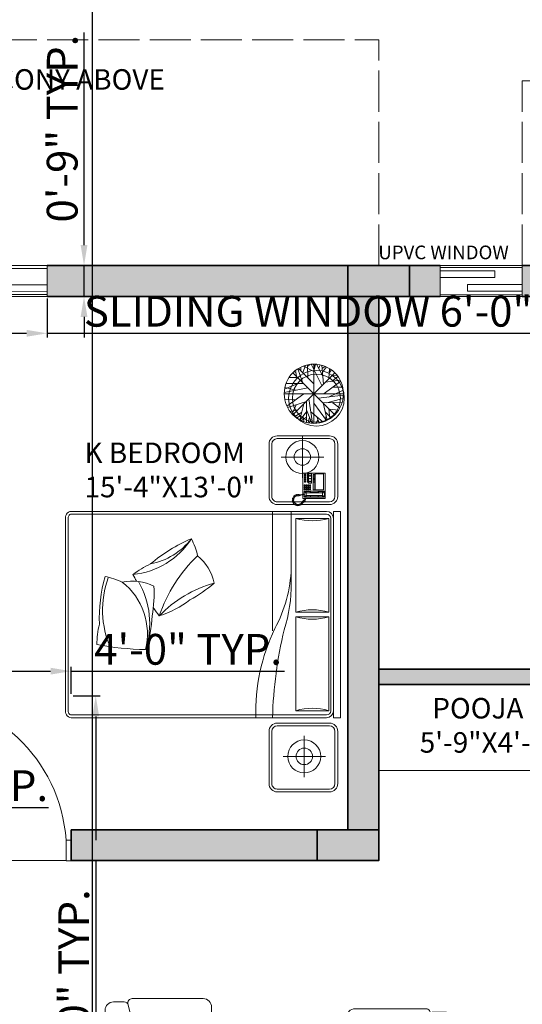
# Model space of a CAD drawing. Units: millimetres. Extents: x 595116 to 630915, y 909473 to 920225.
# Tile 123 of 134: x 629490 to 629637, y 919742 to 920030. Entities that reach past the tile are written whole.
import ezdxf

# ---------------------------------------------------------------- set-up
doc = ezdxf.new("R2010")
doc.units = ezdxf.units.MM
doc.linetypes.add('ACAD_ISO02W100', pattern=[15, 12, -3])
for name, color, linetype, lineweight in [('A-AREA-IDEN', 7, 'Continuous', 20), ('A-FLOR-OVHD', 253, 'ACAD_ISO02W100', 13), ('A-FURN', 32, 'Continuous', 18), ('A-WALL', 1, 'Continuous', 35), ('A-WALL-PATT', 8, 'Continuous', 13), ('Column', 6, 'Continuous', 35), ('Dimension', 3, 'Continuous', 18), ('Doors', 31, 'Continuous', 20), ('L-PLNT', 85, 'Continuous', 13), ('Text', 7, 'Continuous', 18), ('Windows', 33, 'Continuous', 18)]:
    doc.layers.add(name, color=color, linetype=linetype, lineweight=lineweight)
doc.styles.get("Standard").update_dxf_attribs({"font": 'arial.ttf'})
doc.dimstyles.new('ISO-25', dxfattribs={"dimtxt": 9, "dimasz": 6, "dimexe": 1.25, "dimexo": 0.625, "dimtad": 1, "dimlunit": 4, "dimtxsty": 'Standard', "dimcen": 2.5, "dimadec": 0, "dimazin": 0, "dimtfac": 1, "dimtmove": 0, "dimatfit": 3, "dimfxl": 1, "dimarcsym": 0})

# ---------------------------------------------------------------- blocks, each defined once
blk = doc.blocks.new('KWD')
for points in [[(629753.63, 919957.93), (629752.54, 919957.93), (629752.54, 919953.43), (629753.63, 919953.43)], [(629787.45, 919957.93), (629787.45, 919953.43), (629788.54, 919953.43), (629788.54, 919957.93)]]:
    blk.add_lwpolyline(points, close=True)
blk.add_lwpolyline([(629753.63, 919921.79), (629753.63, 919955.68), (629754.13, 919955.68), (629754.13, 919921.8)])
blk.add_arc((629753.64, 919955.68), 33.88, 269.99, 356.196)
blk = doc.blocks.new('A$C356F0359')
for p, q in [((0.4398, 1.9801), (0.0598, 1.9801)), ((0.4398, 1.9601), (0.0598, 1.9601)), ((0.5489, 2), (2.0492, 2)), ((0.5489, 1.9489), (0.5489, 2)), ((2.0492, 1.9489), (0.5489, 1.9489)), ((2.0492, 1.9489), (2.0492, 2)), ((2.5283, 1.9801), (2.1483, 1.9801)), ((2.5283, 1.9601), (2.1483, 1.9601)), ((-0.0002, 1.9201), (-0.0002, 1.5401)), ((0.0198, 1.9201), (0.0198, 1.5401)), ((0.1539, 1.5681), (0.1539, 1.8777)), ((0.2725, 1.8879), (0.2702, 1.8856)), ((0.2702, 1.8856), (0.2702, 1.7279)), ((0.2725, 1.8879), (0.4531, 1.8879)), ((0.3913, 1.8753), (0.277, 1.8753)), ((0.277, 1.8753), (0.277, 1.8147)), ((0.3913, 1.8147), (0.3913, 1.8753)), ((0.4016, 1.8787), (0.4062, 1.8845)), ((0.4016, 1.7404), (0.4016, 1.8787)), ((0.4062, 1.881), (0.405, 1.8765)), ((0.405, 1.8765), (0.4153, 1.8662)), ((0.405, 1.8765), (0.405, 1.8456)), ((0.4062, 1.8845), (0.4405, 1.8845)), ((0.4108, 1.8833), (0.4062, 1.881)), ((0.4108, 1.8833), (0.4382, 1.8833)), ((0.4165, 1.8685), (0.4108, 1.8833)), ((0.4153, 1.8662), (0.4165, 1.8685)), ((0.4153, 1.8147), (0.4153, 1.8662)), ((0.4325, 1.8685), (0.4165, 1.8685)), ((0.4325, 1.8685), (0.4382, 1.8833)), ((0.4336, 1.8662), (0.4325, 1.8685)), ((0.4439, 1.8765), (0.4336, 1.8662)), ((0.4336, 1.8147), (0.4336, 1.8662)), ((0.4382, 1.8833), (0.4428, 1.881)), ((0.4405, 1.8845), (0.4462, 1.8787)), ((0.4428, 1.881), (0.4439, 1.8765)), ((0.4439, 1.8765), (0.4439, 1.8456)), ((0.4462, 1.8787), (0.4462, 1.7416)), ((0.4531, 1.8879), (0.4553, 1.8856)), ((0.4553, 1.8856), (0.4553, 1.7279)), ((0.4798, 1.5401), (0.4798, 1.9201)), ((0.4998, 1.5401), (0.4998, 1.9201)), ((0.5489, 1.8977), (0.5489, 0.0512)), ((0.5689, 1.8977), (0.5689, 0.0512)), ((1.998, 1.9289), (0.6001, 1.9289)), ((2.0292, 0.0512), (2.0292, 1.8977)), ((2.0492, 0.0512), (2.0492, 1.8977)), ((2.0883, 1.9201), (2.0883, 1.5401)), ((2.1083, 1.9201), (2.1083, 1.5401)), ((2.3306, 1.5822), (2.3306, 1.8917)), ((2.5683, 1.5401), (2.5683, 1.9201)), ((2.5883, 1.5401), (2.5883, 1.9201)), ((0.277, 1.8147), (0.3913, 1.8147)), ((0.3913, 1.8125), (0.2816, 1.8125)), ((0.2816, 1.8125), (0.2816, 1.801)), ((0.2816, 1.801), (0.3913, 1.801)), ((0.2907, 1.8125), (0.2907, 1.801)), ((0.2999, 1.8125), (0.2999, 1.801)), ((0.309, 1.8125), (0.309, 1.801)), ((0.3182, 1.8125), (0.3182, 1.801)), ((0.3273, 1.8125), (0.3273, 1.801)), ((0.3365, 1.8125), (0.3365, 1.801)), ((0.3913, 1.801), (0.3913, 1.8125)), ((0.405, 1.8456), (0.4073, 1.8399)), ((0.4073, 1.8399), (0.4108, 1.8342)), ((0.4108, 1.8342), (0.4119, 1.8262)), ((0.4108, 1.785), (0.4119, 1.793)), ((0.4119, 1.8262), (0.4119, 1.8147)), ((0.4119, 1.793), (0.4119, 1.8147)), ((0.4153, 1.8147), (0.4153, 1.753)), ((0.4336, 1.8147), (0.4336, 1.753)), ((0.4382, 1.8342), (0.4371, 1.8262)), ((0.4371, 1.8262), (0.4371, 1.8147)), ((0.4371, 1.793), (0.4371, 1.8147)), ((0.4382, 1.785), (0.4371, 1.793)), ((0.4416, 1.8399), (0.4382, 1.8342)), ((0.4439, 1.8456), (0.4416, 1.8399)), ((0.3052, 1.7226), (0.0051, 1.7226)), ((0.2702, 1.7279), (0.2725, 1.7256)), ((0.4244, 1.7256), (0.2725, 1.7256)), ((0.277, 1.7885), (0.277, 1.7679)), ((0.3445, 1.7885), (0.277, 1.7885)), ((0.277, 1.7679), (0.3445, 1.7679)), ((0.2782, 1.7622), (0.2782, 1.7576)), ((0.2896, 1.7622), (0.2782, 1.7622)), ((0.2782, 1.7576), (0.2896, 1.7576)), ((0.2782, 1.745), (0.2896, 1.745)), ((0.2782, 1.7382), (0.2782, 1.745)), ((0.2896, 1.7382), (0.2782, 1.7382)), ((0.2885, 1.7862), (0.2885, 1.7827)), ((0.2919, 1.7862), (0.2885, 1.7862)), ((0.2885, 1.7827), (0.2919, 1.7827)), ((0.2919, 1.7736), (0.2885, 1.7736)), ((0.2885, 1.7736), (0.2885, 1.7702)), ((0.2885, 1.7702), (0.2919, 1.7702)), ((0.2896, 1.7576), (0.2896, 1.7622)), ((0.2896, 1.745), (0.2896, 1.7382)), ((0.2919, 1.7827), (0.2919, 1.7862)), ((0.2919, 1.7702), (0.2919, 1.7736)), ((0.2942, 1.7622), (0.2942, 1.7576)), ((0.3056, 1.7622), (0.2942, 1.7622)), ((0.2942, 1.7576), (0.3056, 1.7576)), ((0.2942, 1.745), (0.3056, 1.745)), ((0.2942, 1.7382), (0.2942, 1.745)), ((0.3056, 1.7382), (0.2942, 1.7382)), ((0.3056, 1.7576), (0.3056, 1.7622)), ((0.3056, 1.745), (0.3056, 1.7382)), ((0.3125, 1.7862), (0.309, 1.7862)), ((0.309, 1.7862), (0.309, 1.7827)), ((0.309, 1.7827), (0.3125, 1.7827)), ((0.3125, 1.7736), (0.309, 1.7736)), ((0.309, 1.7736), (0.309, 1.7702)), ((0.309, 1.7702), (0.3125, 1.7702)), ((0.3102, 1.7622), (0.3102, 1.7576)), ((0.3216, 1.7622), (0.3102, 1.7622)), ((0.3102, 1.7576), (0.3216, 1.7576)), ((0.3102, 1.745), (0.3216, 1.745)), ((0.3102, 1.7382), (0.3102, 1.745)), ((0.3216, 1.7382), (0.3102, 1.7382)), ((0.3125, 1.7827), (0.3125, 1.7862)), ((0.3125, 1.7702), (0.3125, 1.7736)), ((0.3216, 1.7576), (0.3216, 1.7622)), ((0.3216, 1.745), (0.3216, 1.7382)), ((0.3376, 1.7622), (0.3262, 1.7622)), ((0.3262, 1.7622), (0.3262, 1.7576)), ((0.3262, 1.7576), (0.3376, 1.7576)), ((0.3262, 1.7382), (0.3262, 1.745)), ((0.3262, 1.745), (0.3376, 1.745)), ((0.3376, 1.7382), (0.3262, 1.7382)), ((0.333, 1.7862), (0.3296, 1.7862)), ((0.3296, 1.7862), (0.3296, 1.7827)), ((0.3296, 1.7827), (0.333, 1.7827)), ((0.333, 1.7736), (0.3296, 1.7736)), ((0.3296, 1.7736), (0.3296, 1.7702)), ((0.3296, 1.7702), (0.333, 1.7702)), ((0.333, 1.7827), (0.333, 1.7862)), ((0.333, 1.7702), (0.333, 1.7736)), ((0.3376, 1.7576), (0.3376, 1.7622)), ((0.3376, 1.745), (0.3376, 1.7382)), ((0.3445, 1.7679), (0.3445, 1.7885)), ((0.3548, 1.7759), (0.3548, 1.7827)), ((0.3548, 1.7827), (0.3639, 1.7827)), ((0.3639, 1.7759), (0.3548, 1.7759)), ((0.3548, 1.7633), (0.3548, 1.7702)), ((0.3548, 1.7702), (0.3639, 1.7702)), ((0.3639, 1.7633), (0.3548, 1.7633)), ((0.3548, 1.7564), (0.3639, 1.7564)), ((0.3548, 1.7496), (0.3548, 1.7564)), ((0.3639, 1.7496), (0.3548, 1.7496)), ((0.3548, 1.737), (0.3548, 1.7439)), ((0.3548, 1.7439), (0.3639, 1.7439)), ((0.3639, 1.737), (0.3548, 1.737)), ((0.3639, 1.7827), (0.3639, 1.7759)), ((0.3639, 1.7702), (0.3639, 1.7633)), ((0.3639, 1.7564), (0.3639, 1.7496)), ((0.3639, 1.7439), (0.3639, 1.737)), ((0.3685, 1.7827), (0.3776, 1.7827)), ((0.3685, 1.7759), (0.3685, 1.7827)), ((0.3776, 1.7759), (0.3685, 1.7759)), ((0.3685, 1.7633), (0.3685, 1.7702)), ((0.3685, 1.7702), (0.3776, 1.7702)), ((0.3776, 1.7633), (0.3685, 1.7633)), ((0.3685, 1.7564), (0.3776, 1.7564)), ((0.3685, 1.7496), (0.3685, 1.7564)), ((0.3776, 1.7496), (0.3685, 1.7496)), ((0.3685, 1.737), (0.3685, 1.7439)), ((0.3685, 1.7439), (0.3776, 1.7439)), ((0.3776, 1.737), (0.3685, 1.737)), ((0.3776, 1.7827), (0.3776, 1.7759)), ((0.3776, 1.7702), (0.3776, 1.7633)), ((0.3776, 1.7564), (0.3776, 1.7496)), ((0.3776, 1.7439), (0.3776, 1.737)), ((0.3822, 1.7759), (0.3822, 1.7827)), ((0.3822, 1.7827), (0.3913, 1.7827)), ((0.3913, 1.7759), (0.3822, 1.7759)), ((0.3822, 1.7633), (0.3822, 1.7702)), ((0.3822, 1.7702), (0.3913, 1.7702)), ((0.3913, 1.7633), (0.3822, 1.7633)), ((0.3822, 1.7576), (0.3913, 1.7576)), ((0.3822, 1.7507), (0.3822, 1.7576)), ((0.3913, 1.7507), (0.3822, 1.7507)), ((0.3822, 1.7439), (0.3913, 1.7439)), ((0.3822, 1.737), (0.3822, 1.7439)), ((0.3913, 1.737), (0.3822, 1.737)), ((0.3913, 1.7827), (0.3913, 1.7759)), ((0.3913, 1.7702), (0.3913, 1.7633)), ((0.3913, 1.7576), (0.3913, 1.7507)), ((0.3913, 1.7439), (0.3913, 1.737)), ((0.4073, 1.7347), (0.4016, 1.7404)), ((0.405, 1.7736), (0.4073, 1.7793)), ((0.405, 1.7427), (0.405, 1.7736)), ((0.405, 1.7427), (0.4153, 1.753)), ((0.4062, 1.7382), (0.405, 1.7427)), ((0.4108, 1.7359), (0.4062, 1.7382)), ((0.4073, 1.7793), (0.4108, 1.785)), ((0.4234, 1.7347), (0.4073, 1.7347)), ((0.4165, 1.7507), (0.4108, 1.7359)), ((0.4108, 1.7359), (0.4234, 1.7359)), ((0.4153, 1.753), (0.4165, 1.7507)), ((0.4325, 1.7507), (0.4165, 1.7507)), ((0.4233, 1.7393), (0.4235, 1.7294)), ((0.4268, 1.7393), (0.4233, 1.7393)), ((0.4235, 1.7294), (0.4263, 1.7179)), ((0.4274, 1.7301), (0.4268, 1.7393)), ((0.427, 1.7359), (0.4382, 1.7359)), ((0.4405, 1.7347), (0.4271, 1.7347)), ((0.429, 1.7227), (0.4274, 1.7301)), ((0.4531, 1.7256), (0.4284, 1.7256)), ((0.4318, 1.7119), (0.429, 1.7227)), ((0.4336, 1.753), (0.4325, 1.7507)), ((0.4325, 1.7507), (0.4382, 1.7359)), ((0.4439, 1.7427), (0.4336, 1.753)), ((0.4416, 1.7793), (0.4382, 1.785)), ((0.4382, 1.7359), (0.4428, 1.7382)), ((0.4462, 1.7416), (0.4405, 1.7347)), ((0.4439, 1.7736), (0.4416, 1.7793)), ((0.4428, 1.7382), (0.4439, 1.7427)), ((0.4439, 1.7427), (0.4439, 1.7736)), ((0.4553, 1.7279), (0.4531, 1.7256)), ((0.4622, 1.7459), (0.4553, 1.7484)), ((0.4553, 1.7439), (0.4604, 1.7425)), ((0.4604, 1.7425), (0.465, 1.7388)), ((0.4654, 1.7427), (0.4622, 1.7459)), ((0.465, 1.7388), (0.4662, 1.7372)), ((0.4678, 1.7405), (0.4654, 1.7427)), ((0.4662, 1.7372), (0.4686, 1.7374)), ((0.4686, 1.7374), (0.4662, 1.735)), ((0.4662, 1.735), (0.4755, 1.7268)), ((0.4721, 1.7421), (0.4678, 1.7405)), ((0.4741, 1.7401), (0.4721, 1.7421)), ((0.4725, 1.7366), (0.4741, 1.7401)), ((0.4753, 1.7388), (0.4725, 1.7366)), ((0.4783, 1.7356), (0.4753, 1.7388)), ((0.4755, 1.7268), (0.4906, 1.7139)), ((0.4759, 1.729), (0.4783, 1.7356)), ((0.4821, 1.7322), (0.4759, 1.729)), ((0.4874, 1.7272), (0.4821, 1.7322)), ((0.4862, 1.7199), (0.4874, 1.7272)), ((0.4914, 1.7231), (0.4862, 1.7199)), ((0.4958, 1.7185), (0.4914, 1.7231)), ((0.494, 1.7135), (0.4958, 1.7185)), ((2.4819, 1.7366), (2.1818, 1.7366)), ((0.4263, 1.7179), (0.429, 1.707)), ((0.427, 1.697), (0.4265, 1.6915)), ((0.4265, 1.6915), (0.4332, 1.6903)), ((0.4332, 1.6903), (0.4267, 1.6864)), ((0.4267, 1.6864), (0.4272, 1.6801)), ((0.4295, 1.6996), (0.427, 1.697)), ((0.4272, 1.6801), (0.4346, 1.6794)), ((0.4346, 1.6794), (0.4281, 1.6744)), ((0.4281, 1.6744), (0.4311, 1.669)), ((0.429, 1.707), (0.4288, 1.701)), ((0.4288, 1.701), (0.4295, 1.6996)), ((0.4311, 1.669), (0.4381, 1.6704)), ((0.4325, 1.7063), (0.4318, 1.7119)), ((0.4323, 1.7003), (0.4325, 1.7063)), ((0.4364, 1.6973), (0.4323, 1.7003)), ((0.4381, 1.6704), (0.4348, 1.6639)), ((0.4348, 1.6639), (0.4383, 1.6598)), ((0.4355, 1.6919), (0.4364, 1.6973)), ((0.4367, 1.6774), (0.4355, 1.6919)), ((0.4455, 1.6663), (0.4367, 1.6774)), ((0.4383, 1.6598), (0.4436, 1.6637)), ((0.4436, 1.6637), (0.4427, 1.6575)), ((0.4427, 1.6575), (0.4471, 1.6547)), ((0.4577, 1.6598), (0.4455, 1.6663)), ((0.4471, 1.6547), (0.4526, 1.6593)), ((0.4526, 1.6593), (0.4519, 1.6517)), ((0.4519, 1.6517), (0.4568, 1.6503)), ((0.4568, 1.6503), (0.4598, 1.6565)), ((0.4716, 1.6586), (0.4577, 1.6598)), ((0.4598, 1.6565), (0.4626, 1.6503)), ((0.4626, 1.6503), (0.4665, 1.6498)), ((0.4665, 1.6498), (0.4681, 1.6565)), ((0.4681, 1.6565), (0.4707, 1.6491)), ((0.4707, 1.6491), (0.4751, 1.6503)), ((0.485, 1.6644), (0.4716, 1.6586)), ((0.4751, 1.6503), (0.4753, 1.6565)), ((0.4753, 1.6565), (0.4806, 1.6519)), ((0.4806, 1.6519), (0.4843, 1.6538)), ((0.4843, 1.6538), (0.4836, 1.6607)), ((0.4836, 1.6607), (0.4885, 1.6547)), ((0.4952, 1.6744), (0.485, 1.6644)), ((0.4885, 1.6547), (0.4922, 1.6579)), ((0.4922, 1.6579), (0.4894, 1.6642)), ((0.4894, 1.6642), (0.4959, 1.6614)), ((0.4908, 1.7135), (0.4984, 1.6917)), ((0.501, 1.7142), (0.494, 1.7135)), ((0.4984, 1.6917), (0.4952, 1.6744)), ((0.4957, 1.6704), (0.5024, 1.6683)), ((0.4989, 1.6642), (0.4957, 1.6704)), ((0.4959, 1.6614), (0.4989, 1.6642)), ((0.4964, 1.7047), (0.5031, 1.7072)), ((0.5038, 1.7049), (0.4964, 1.7047)), ((0.5042, 1.673), (0.4987, 1.6792)), ((0.4987, 1.6792), (0.5058, 1.679)), ((0.5005, 1.695), (0.5054, 1.6996)), ((0.5068, 1.695), (0.5005, 1.695)), ((0.5008, 1.6871), (0.5079, 1.6892)), ((0.5068, 1.6836), (0.5008, 1.6871)), ((0.5031, 1.7072), (0.501, 1.7142)), ((0.5024, 1.6683), (0.5042, 1.673)), ((0.5054, 1.6996), (0.5038, 1.7049)), ((0.5058, 1.679), (0.5068, 1.6836)), ((0.5079, 1.6892), (0.5068, 1.695)), ((0.0598, 1.5001), (0.4398, 1.5001)), ((0.0598, 1.4801), (0.4398, 1.4801)), ((2.1483, 1.5001), (2.5283, 1.5001)), ((2.1483, 1.4801), (2.5283, 1.4801)), ((0.6001, 0.02), (1.998, 0.02)), ((0.6001, 0), (1.998, 0))]:
    blk.add_line(p, q)
at = {"linetype": 'ByBlock'}
for p, q in [((0.6001, 1.9147), (1.282, 1.9147)), ((0.6001, 1.6759), (0.6001, 1.9147)), ((1.282, 1.9147), (1.282, 1.6759)), ((1.3161, 1.9147), (1.998, 1.9147)), ((1.3161, 1.6759), (1.3161, 1.9147)), ((1.998, 1.9147), (1.998, 1.6759)), ((1.282, 1.6759), (0.6001, 1.6759)), ((1.998, 1.6759), (1.3161, 1.6759)), ((1.0687, 1.6418), (0.5489, 1.6418)), ((1.4185, 1.5053), (0.5489, 1.5053))]:
    blk.add_line(p, q, dxfattribs=at)
for centre in [(0.1539, 1.7226), (2.3306, 1.7366)]:
    blk.add_circle(centre, 0.12, dxfattribs=at)
for centre in [(2.3306, 1.7366), (0.1539, 1.7226)]:
    blk.add_circle(centre, 0.06)
for centre, radius, start, end in [((0.0598, 1.9201), 0.06, 90, 180), ((0.0598, 1.9201), 0.04, 90, 180), ((0.4398, 1.9201), 0.06, 0, 90), ((0.4398, 1.9201), 0.04, 0, 90), ((0.6001, 1.8977), 0.0512, 90, 180), ((1.998, 1.8977), 0.0512, 0, 90), ((2.1483, 1.9201), 0.06, 90, 180), ((2.1483, 1.9201), 0.04, 90, 180), ((2.5283, 1.9201), 0.06, 0, 90), ((2.5283, 1.9201), 0.04, 0, 90), ((0.6001, 1.8977), 0.0312, 90, 180), ((1.998, 1.8977), 0.0312, 0, 90), ((0.0598, 1.5401), 0.06, 180, 270), ((0.0598, 1.5401), 0.04, 180, 270), ((0.4398, 1.5401), 0.04, 270, 0), ((0.4398, 1.5401), 0.06, 270, 0), ((2.1483, 1.5401), 0.06, 180, 270), ((2.1483, 1.5401), 0.04, 180, 270), ((2.5283, 1.5401), 0.06, 270, 0), ((2.5283, 1.5401), 0.04, 270, 0), ((1.1471, 0.7332), 0.3575, 102.47819, 140.46254), ((1.9086, 1.3124), 0.8697, 195.33601, 226.41927), ((0.3249, 0.4335), 0.9879, 28.49711, 41.05657), ((0.9965, 0.4273), 0.548, 103.20343, 117.03623), ((1.6529, 1.7059), 1.0798, 223.63057, 251.4288), ((0.4451, 0.4375), 0.5655, 5.33912, 57.68949), ((0.4517, 0.5274), 0.4879, 10.69865, 52.68638), ((1.8195, 1.3719), 1.1652, 203.06416, 220.32086), ((0.5617, 0.4344), 0.7874, 18.35266, 36.68512), ((1.1372, -0.3434), 0.9879, 80.06073, 92.62018), ((-0.021, 2.4319), 2.1977, 305.29657, 307.24182), ((1.5949, 0.9312), 0.734, 205.25901, 216.93514), ((1.4135, 0.487), 0.3575, 154.0418, 192.02615), ((1.3641, 0.0041), 0.6085, 71.81005, 120.13512), ((1.44, 0.1186), 0.4774, 76.18494, 142.00166), ((1.2836, -0.1573), 0.7874, 69.91627, 88.24873), ((-0.6432, 0.628), 2.1977, 349.48843, 358.80544), ((-0.021, 2.4319), 2.1977, 297.92482, 299.3793), ((1.5595, 0.1789), 0.548, 154.76704, 168.59984), ((1.3312, 1.4107), 1.1652, 254.62778, 271.88448), ((1.2647, 0.9578), 0.6885, 250.29361, 293.6414), ((1.5368, 0.9609), 0.734, 256.82263, 268.49876), ((0.5943, 0.0454), 0.0458, 172.75992, 277.24008), ((0.5943, 0.0454), 0.0258, 172.75992, 277.24008), ((2.0038, 0.0454), 0.0458, 262.75992, 7.24008), ((2.0038, 0.0454), 0.0258, 262.75992, 7.24008)]:
    blk.add_arc(centre, radius, start, end)
for centre, radius, start, end in [((0.1906, 1.7953), 0.4265, 343.73979, 16.26021), ((1.6914, 1.7953), 0.4265, 163.73979, 196.26021), ((0.9067, 1.7953), 0.4265, 343.73979, 16.26021), ((2.4075, 1.7953), 0.4265, 163.73979, 196.26021), ((0.9303, 0.657), 0.9853, 61.43285, 88.12613), ((1.0826, 0.5712), 1.0706, 72.19663, 90.74184), ((2.1368, 4.5996), 3.0955, 256.42012, 268.37887), ((2.0056, 2.7745), 1.3903, 244.24266, 271.79845)]:
    blk.add_arc(centre, radius, start, end, dxfattribs=at)
blk = doc.blocks.new('SOFA')
for p, q in [((629543.7, 919743.59), (629522.89, 919743.59)), ((629522.89, 919743.59), (629543.7, 919743.59)), ((629520.59, 919742.63), (629517.45, 919742.63)), ((629517.45, 919742.63), (629520.59, 919742.63)), ((629521.79, 919741.7), (629521.7, 919742.06)), ((629521.7, 919742.06), (629523.2, 919736.06)), ((629546.16, 919741.12), (629546.16, 919739.22)), ((629546.16, 919741.12), (629546.16, 919737.29)), ((629588.11, 919740.62), (629608.91, 919740.62)), ((629588.11, 919740.62), (629608.91, 919740.62)), ((629514.98, 919740.17), (629514.98, 919695.65)), ((629514.98, 919695.65), (629514.98, 919740.17)), ((629547.17, 919738.01), (629547.17, 919695.65)), ((629547.17, 919738.01), (629547.17, 919695.65)), ((629585.64, 919738.15), (629585.64, 919734.33)), ((629585.64, 919736.25), (629585.64, 919738.15)), ((629610.11, 919739.09), (629608.61, 919733.09)), ((629610.11, 919739.09), (629610.02, 919738.73)), ((629611.21, 919739.66), (629614.36, 919739.66)), ((629611.21, 919739.66), (629614.36, 919739.66)), ((629523.2, 919736.06), (629523.2, 919695.65)), ((629523.2, 919695.65), (629523.2, 919736.06)), ((629523.2, 919695.65), (629523.2, 919736.06)), ((629544.93, 919736.06), (629523.2, 919736.06)), ((629523.2, 919736.06), (629523.53, 919736.06)), ((629523.2, 919736.06), (629523.53, 919736.06)), ((629523.53, 919736.06), (629523.53, 919695.65)), ((629523.53, 919736.06), (629523.53, 919695.65)), ((629523.53, 919736.06), (629523.53, 919695.65)), ((629584.64, 919735.04), (629584.64, 919712.53)), ((629584.64, 919712.53), (629584.64, 919735.04)), ((629616.82, 919737.2), (629616.82, 919710.3)), ((629616.82, 919737.2), (629616.82, 919710.3)), ((629586.87, 919733.09), (629608.61, 919733.09)), ((629608.28, 919733.09), (629608.61, 919733.09)), ((629608.28, 919714.4), (629608.28, 919733.09)), ((629608.28, 919733.09), (629608.28, 919714.4)), ((629608.61, 919733.09), (629608.61, 919714.4)), ((629608.61, 919733.09), (629608.61, 919714.4)), ((629556.25, 919728.06), (629556.25, 919687.01)), ((629556.25, 919687.01), (629556.25, 919728.06)), ((629576.77, 919728.06), (629556.25, 919728.06)), ((629556.25, 919728.06), (629576.77, 919728.06)), ((629559.82, 919728), (629559.82, 919727.13)), ((629561.06, 919728), (629561.06, 919725.63)), ((629562.29, 919728), (629562.29, 919724.5)), ((629563.52, 919728), (629563.52, 919723.63)), ((629564.75, 919728), (629564.75, 919722.96)), ((629565.98, 919728), (629565.98, 919722.42)), ((629567.19, 919727.97), (629567.19, 919721.68)), ((629568.42, 919727.08), (629568.42, 919720.54)), ((629576.77, 919687.01), (629576.77, 919728.06)), ((629576.77, 919728.06), (629576.77, 919687.01)), ((629569.65, 919725.8), (629569.65, 919718.67)), ((629569.65, 919725.8), (629569.65, 919718.67)), ((629570.88, 919723.75), (629570.88, 919716.49)), ((629570.88, 919716.49), (629570.88, 919723.75)), ((629572.12, 919720.99), (629572.12, 919714.94)), ((629573.35, 919718.86), (629573.35, 919713.74)), ((629547.17, 919715.59), (629514.98, 919715.59)), ((629574.58, 919717.12), (629574.58, 919712.78)), ((629575.81, 919715.64), (629575.81, 919712.02)), ((629586.87, 919714.4), (629608.61, 919714.4)), ((629608.61, 919714.4), (629608.28, 919714.4)), ((629610.09, 919708.48), (629608.61, 919714.4)), ((629557.33, 919712.4), (629557.33, 919707.56)), ((629557.33, 919707.56), (629557.33, 919712.4)), ((629585.64, 919709.42), (629585.64, 919713.17)), ((629558.57, 919711.23), (629558.57, 919706.97)), ((629559.8, 919710.18), (629559.8, 919706.31)), ((629561.03, 919709.25), (629561.03, 919705.57)), ((629585.64, 919709.42), (629585.64, 919711.32)), ((629610.02, 919708.77), (629610.09, 919708.48)), ((629562.26, 919708.41), (629562.26, 919704.73)), ((629563.49, 919707.66), (629563.49, 919703.8)), ((629564.72, 919706.99), (629564.72, 919702.74)), ((629565.96, 919706.31), (629565.96, 919701.75)), ((629588.11, 919706.95), (629608.89, 919706.95)), ((629608.89, 919706.95), (629588.11, 919706.95)), ((629611.21, 919707.83), (629611.48, 919707.83)), ((629611.48, 919707.83), (629611.21, 919707.83)), ((629611.48, 919707.83), (629614.36, 919707.83)), ((629614.36, 919707.83), (629611.48, 919707.83)), ((629567.19, 919705.56), (629567.19, 919701.12)), ((629568.42, 919704.73), (629568.42, 919700.78)), ((629569.65, 919703.81), (629569.65, 919700.45)), ((629570.88, 919702.8), (629570.88, 919699.98)), ((629572.12, 919701.68), (629572.12, 919699.37)), ((629573.35, 919700.43), (629573.35, 919698.59)), ((629574.58, 919699.04), (629574.58, 919697.6)), ((629575.81, 919697.48), (629575.81, 919696.34)), ((629575.81, 919697.48), (629575.81, 919696.34)), ((629547.17, 919695.06), (629514.98, 919695.06)), ((629514.98, 919695.06), (629514.98, 919670.42)), ((629514.98, 919670.42), (629514.98, 919695.06)), ((629514.98, 919695.06), (629515.44, 919695.06)), ((629515.6, 919695.04), (629546.55, 919695.04)), ((629523.2, 919695.06), (629523.2, 919674.53)), ((629523.2, 919674.53), (629523.2, 919695.04)), ((629523.2, 919674.53), (629523.2, 919695.04)), ((629523.2, 919695.04), (629523.53, 919695.04)), ((629523.2, 919695.04), (629523.53, 919695.04)), ((629523.53, 919695.04), (629523.53, 919695.11)), ((629523.53, 919695.04), (629523.53, 919695.11)), ((629523.53, 919695.06), (629523.53, 919674.53)), ((629523.53, 919695.04), (629523.53, 919674.53)), ((629523.53, 919695.04), (629523.53, 919674.53)), ((629524.14, 919695.04), (629523.53, 919695.04)), ((629524.14, 919695.04), (629523.53, 919695.04)), ((629546.71, 919695.06), (629547.17, 919695.06)), ((629547.17, 919695.06), (629547.17, 919672.66)), ((629547.17, 919695.06), (629547.17, 919672.66)), ((629588.11, 919692.76), (629608.89, 919692.76)), ((629608.89, 919692.76), (629588.11, 919692.76)), ((629611.21, 919691.88), (629611.48, 919691.88)), ((629611.48, 919691.88), (629611.21, 919691.88)), ((629611.48, 919691.88), (629614.36, 919691.88)), ((629614.36, 919691.88), (629611.48, 919691.88)), ((629585.64, 919690.3), (629585.64, 919688.39)), ((629585.64, 919690.3), (629585.64, 919686.55)), ((629610.09, 919691.23), (629608.61, 919685.31)), ((629610.02, 919690.95), (629610.09, 919691.23)), ((629616.82, 919662.52), (629616.82, 919689.42)), ((629616.82, 919662.52), (629616.82, 919689.42)), ((629556.25, 919687.01), (629576.77, 919687.01)), ((629576.77, 919687.01), (629556.25, 919687.01)), ((629584.64, 919664.68), (629584.64, 919687.18)), ((629584.64, 919687.18), (629584.64, 919664.68)), ((629586.87, 919685.31), (629608.61, 919685.31)), ((629608.61, 919685.31), (629608.28, 919685.31)), ((629608.28, 919685.31), (629608.28, 919666.62)), ((629608.28, 919666.62), (629608.28, 919685.31)), ((629608.61, 919666.62), (629608.61, 919685.31)), ((629608.61, 919666.62), (629608.61, 919685.31)), ((629521.72, 919668.61), (629523.2, 919674.53)), ((629544.93, 919674.53), (629523.2, 919674.53)), ((629523.53, 919674.53), (629523.2, 919674.53)), ((629523.53, 919674.53), (629523.2, 919674.53)), ((629546.16, 919669.54), (629546.16, 919673.3)), ((629546.16, 919671.45), (629546.16, 919669.54)), ((629521.72, 919668.61), (629521.79, 919668.89)), ((629520.32, 919667.96), (629517.45, 919667.96)), ((629520.32, 919667.96), (629517.45, 919667.96)), ((629520.59, 919667.96), (629520.32, 919667.96)), ((629520.59, 919667.96), (629520.32, 919667.96)), ((629543.7, 919667.08), (629522.91, 919667.08)), ((629543.7, 919667.08), (629522.91, 919667.08)), ((629585.64, 919661.56), (629585.64, 919665.39)), ((629586.87, 919666.62), (629608.61, 919666.62)), ((629608.28, 919666.62), (629608.61, 919666.62)), ((629610.11, 919660.63), (629608.61, 919666.62)), ((629585.64, 919663.47), (629585.64, 919661.56)), ((629610.11, 919660.63), (629610.02, 919660.99)), ((629611.21, 919660.05), (629614.36, 919660.05)), ((629611.21, 919660.05), (629614.36, 919660.05)), ((629588.11, 919659.1), (629608.91, 919659.1)), ((629588.11, 919659.1), (629608.91, 919659.1))]:
    blk.add_line(p, q)
for centre, radius, start, end in [((629522.89, 919742.36), 1.23, 90, 194.0362), ((629522.89, 919742.36), 1.23, 90, 194.0362), ((629543.7, 919741.12), 2.46, 0, 90), ((629543.7, 919741.12), 2.46, 0, 90), ((629517.45, 919740.17), 2.46, 90, 180), ((629517.45, 919740.17), 2.46, 90, 180), ((629520.59, 919741.4), 1.23, 14.0362, 90), ((629520.59, 919741.4), 1.23, 14.0362, 90), ((629588.11, 919738.15), 2.46, 90, 180), ((629588.11, 919738.15), 2.46, 90, 180), ((629608.91, 919739.39), 1.23, 345.9638, 90), ((629608.91, 919739.39), 1.23, 345.9638, 90), ((629545.94, 919738.01), 1.23, 0, 90), ((629545.94, 919738.01), 1.23, 0, 79.4007), ((629611.21, 919738.43), 1.23, 90, 165.9638), ((629611.21, 919738.43), 1.23, 90, 165.9638), ((629614.36, 919737.2), 2.46, 0, 90), ((629614.36, 919737.2), 2.46, 0, 90), ((629544.93, 919737.29), 1.23, 270, 0), ((629585.87, 919735.04), 1.23, 90, 180), ((629585.87, 919735.04), 1.23, 100.5993, 180), ((629586.87, 919734.33), 1.23, 180, 270), ((629570.11, 919734.3), 12.54, 210.2644, 248.0021), ((629562.37, 919720.03), 9.29, 21.2599, 58.8091), ((629562.37, 919720.03), 9.29, 23.6102, 38.4008), ((629594.57, 919732.56), 25.26, 201.2599, 225.1217), ((629562.42, 919715.26), 7.99, 24.8088, 68.0021), ((629582.84, 919724.7), 14.51, 204.5645, 214.4539), ((629582.84, 919724.7), 14.51, 204.8088, 245.1378), ((629586.87, 919713.17), 1.23, 90, 180), ((629577.93, 919732.79), 28.98, 222.2366, 242.5747), ((629577.93, 919732.79), 28.98, 224.7026, 242.5747), ((629585.87, 919712.53), 1.23, 180, 270), ((629585.87, 919712.53), 1.23, 180, 259.4007), ((629588.11, 919709.42), 2.46, 180, 270), ((629588.11, 919709.42), 2.46, 180, 270), ((629611.21, 919709.06), 1.23, 194.0362, 270), ((629611.21, 919709.06), 1.23, 194.0362, 270), ((629614.36, 919710.3), 2.46, 270, 0), ((629614.36, 919710.3), 2.46, 270, 0), ((629546.11, 919682.25), 27.68, 46.9747, 68.4773), ((629546.11, 919682.25), 27.68, 46.9747, 66.0851), ((629549.56, 919678.1), 32.63, 33.5604, 62.5747), ((629549.56, 919678.1), 32.63, 36.4252, 62.5747), ((629608.89, 919708.18), 1.23, 270, 14.0362), ((629608.89, 919708.18), 1.23, 270, 14.0362), ((629569.57, 919707.39), 6.7, 226.9747, 258.3827), ((629569.57, 919707.39), 6.7, 226.9746, 258.3828), ((629565.49, 919687.55), 13.55, 33.8658, 78.3827), ((629565.49, 919687.55), 13.55, 40.4201, 78.3827), ((629515.6, 919695.65), 0.616, 180, 270), ((629515.6, 919695.65), 0.616, 180, 255.079), ((629523.81, 919695.65), 0.616, 180, 270), ((629523.81, 919695.65), 0.616, 180, 242.2854), ((629523.81, 919695.65), 0.616, 180, 242.2854), ((629524.14, 919695.65), 0.616, 180, 270), ((629524.14, 919695.65), 0.616, 180, 270), ((629524.14, 919695.65), 0.616, 180, 270), ((629546.55, 919695.65), 0.616, 270, 0), ((629546.55, 919695.65), 0.616, 284.921, 0), ((629588.11, 919690.3), 2.46, 90, 180), ((629588.11, 919690.3), 2.46, 90, 180), ((629608.89, 919691.53), 1.23, 345.9638, 90), ((629608.89, 919691.53), 1.23, 345.9638, 90), ((629611.21, 919690.65), 1.23, 90, 165.9638), ((629611.21, 919690.65), 1.23, 90, 165.9638), ((629614.36, 919689.42), 2.46, 0, 90), ((629614.36, 919689.42), 2.46, 0, 90), ((629585.87, 919687.18), 1.23, 90, 180), ((629585.87, 919687.18), 1.23, 100.5993, 180), ((629586.87, 919686.55), 1.23, 180, 270), ((629544.93, 919673.3), 1.23, 0, 90), ((629545.94, 919672.66), 1.23, 270, 0), ((629545.94, 919672.66), 1.23, 280.5993, 0), ((629517.45, 919670.42), 2.46, 180, 270), ((629517.45, 919670.42), 2.46, 180, 270), ((629520.59, 919669.19), 1.23, 270, 345.9638), ((629520.59, 919669.19), 1.23, 270, 345.9638), ((629522.91, 919668.31), 1.23, 165.9638, 270), ((629522.91, 919668.31), 1.23, 165.9638, 270), ((629543.7, 919669.54), 2.46, 270, 0), ((629543.7, 919669.54), 2.46, 270, 0), ((629586.87, 919665.39), 1.23, 90, 180), ((629585.87, 919664.68), 1.23, 180, 270), ((629585.87, 919664.68), 1.23, 180, 259.4007), ((629614.36, 919662.52), 2.46, 270, 0), ((629614.36, 919662.52), 2.46, 270, 0), ((629588.11, 919661.56), 2.46, 180, 270), ((629588.11, 919661.56), 2.46, 180, 270), ((629608.91, 919660.33), 1.23, 270, 14.0362), ((629608.91, 919660.33), 1.23, 270, 14.0362), ((629611.21, 919661.28), 1.23, 194.0362, 270), ((629611.21, 919661.28), 1.23, 194.0362, 270)]:
    blk.add_arc(centre, radius, start, end)
at = {"flags": 9}
for tag in ['XSIZE', 'YSIZE']:
    blk.add_attdef(tag, (629556.25, 919728.06), '', height=0.0205, rotation=270, dxfattribs=at)
blk = doc.blocks.new('POTTED-PLANT')
for p, q in [((5.49, 15.52), (6.28, 17.77)), ((5.61, 17.51), (8.67, 15.94)), ((6.86, 17.38), (7.52, 18.03)), ((6.89, 14.08), (6.86, 17.93)), ((7.9, 18.06), (11.06, 11.86)), ((9.02, 17.38), (8.46, 18.1)), ((8.67, 18.11), (8.67, 0.76)), ((8.74, 16.47), (9.2, 18.06)), ((11.32, 14.57), (9.46, 18.06)), ((10.09, 16.89), (10.53, 17.9)), ((11.52, 12.26), (11.04, 17.77)), ((11.14, 16.82), (12.03, 17.41)), ((11.24, 15.75), (12.36, 17.28)), ((14.75, 15.51), (2.6, 3.36)), ((14.75, 3.36), (2.6, 15.51)), ((2.87, 15.88), (3.4, 15.68)), ((3.32, 16.24), (3.58, 14.57)), ((3.96, 16.73), (5.31, 12.84)), ((4.16, 16.82), (8.64, 12.35)), ((4.85, 16.17), (4.88, 17.22)), ((13.25, 16.79), (13.05, 13.86)), ((13.17, 15.58), (13.86, 16.4)), ((13.91, 13.07), (15.74, 14.51)), ((14.04, 14.8), (15.41, 14.87)), ((4.01, 12.42), (0.12, 10.79)), ((0.57, 12.45), (5.66, 12.45)), ((1.47, 14.18), (3.93, 14.18)), ((16.53, 13.1), (11.7, 9.48)), ((12.05, 12.81), (16.38, 13.4)), ((0, 9.44), (17.35, 9.44)), ((0.04, 9.84), (6.94, 11.18)), ((0.19, 11.28), (3.48, 10.53)), ((0.78, 5.86), (5.74, 9.45)), ((10.02, 8.11), (17.3, 9.03)), ((12.92, 8.47), (17.27, 10.46)), ((14.24, 11.38), (17.09, 11.41)), ((0.22, 7.66), (3.4, 7.75)), ((0.98, 5.47), (6.25, 7.04)), ((3.48, 6.19), (2.31, 3.58)), ((5.79, 6.51), (4.54, 1.82)), ((6.53, 7.26), (6.56, 1.1)), ((7.22, 7.98), (8.31, 0.8)), ((8.67, 6.68), (12.41, 1.65)), ((11.37, 6.74), (12.54, 1.72)), ((11.39, 6.74), (16.97, 6.94)), ((12.49, 6.77), (17.19, 8.01)), ((14.19, 6.81), (16.25, 5.24)), ((3.99, 4.75), (1.72, 4.29)), ((5.1, 3.97), (3.07, 2.83)), ((4.88, 3.09), (3.65, 2.4)), ((6.56, 4.2), (4.67, 1.78)), ((6.56, 4.78), (8.11, 0.84)), ((7.78, 4.2), (11.26, 1.2)), ((11.98, 4.16), (13.78, 2.43)), ((12.26, 2.96), (12, 1.49)), ((13.07, 5.08), (13.35, 2.21)), ((13.22, 4.91), (15.85, 4.62)), ((6.56, 2.6), (5.05, 1.59)), ((5.56, 2.86), (5.79, 1.33)), ((7.45, 2.57), (7.01, 0.97)), ((7.75, 1.82), (7.32, 0.93)), ((9.89, 1.75), (9.23, 0.84)), ((9.53, 2.7), (10.2, 0.97))]:
    blk.add_line(p, q)
for centre, radius in [((8.67, 9.44), 8.67), ((9.43, 8.14), 8.14), ((9.43, 8.14), 7.03)]:
    blk.add_circle(centre, radius)
blk = doc.blocks.new('WIN-SLIDING-6FT')
for p, q in [((0, 0), (0, 9)), ((0, 9), (72, 9)), ((72, 0), (72, 9)), ((0.01, 7.5), (42, 7.41)), ((42, 7.41), (42, 5.41)), ((0, 5.5), (42, 5.41)), ((30, 3.44), (72, 3.35)), ((30, 3.44), (30, 1.44)), ((30, 1.44), (71.99, 1.35)), ((0, 0), (72, 0))]:
    blk.add_line(p, q)
blk.add_lwpolyline([(0, 8.12), (72, 8.12), (72, 0.59), (0, 0.59)], close=True)
blk = doc.blocks.new('WIN-SLIDING-2FT')
for p, q in [((0, 9), (0, 0)), ((0, 9), (24, 9)), ((24, 9), (24, 0)), ((0, 7.5), (16, 7.5)), ((16, 7.5), (16, 5.5)), ((0, 5.5), (16, 5.5)), ((8, 3.5), (24, 3.5)), ((8, 3.5), (8, 1.5)), ((8, 1.5), (24, 1.5)), ((0, 0), (24, 0))]:
    blk.add_line(p, q)
blk.add_lwpolyline([(0, 8.46), (24, 8.46), (24, 0.48), (0, 0.48)], close=True)
blk = doc.blocks.new('COLUMN-RECT-18X9')
h = blk.add_hatch(color=256)
h.dxf.hatch_style = 1
h.paths.add_polyline_path([(18, 9), (0, 9), (0, 0), (18, 0)])
blk.add_lwpolyline([(0, 9), (18, 9), (18, 0), (0, 0)], close=True)
blk = doc.blocks.new('*D162')
at = {"layer": 'Defpoints', "color": 0, "transparency": 16777216}
for p in [(629505.04, 919832.11), (629505.04, 919783.93), (629512.27, 919783.93)]:
    blk.add_point(p, dxfattribs=at)
at = {"layer": 'Dimension', "color": 0, "lineweight": -2, "transparency": 16777216}
for p, q in [((629505.67, 919832.11), (629513.52, 919832.11)), ((629512.27, 919826.11), (629512.27, 919789.93)), ((629505.67, 919783.93), (629513.52, 919783.93)), ((629512.27, 919783.93), (629512.27, 919681.05))]:
    blk.add_line(p, q, dxfattribs=at)
at = {"layer": 'Dimension', "color": 0, "transparency": 16777216}
for points in [[(629511.27, 919826.11), (629513.27, 919826.11), (629512.27, 919832.11)], [(629511.27, 919789.93), (629513.27, 919789.93), (629512.27, 919783.93)]]:
    blk.add_solid(points, dxfattribs=at)
at = {"layer": 'Dimension', "color": 0, "transparency": 16777216, "insert": (629506.99, 919729.49), "char_height": 9, "attachment_point": 5, "rotation": 90}
blk.add_mtext('DOOR 4\'-0" TYP.', dxfattribs=at)
blk = doc.blocks.new('*D163')
at = {"layer": 'Defpoints', "color": 0, "transparency": 16777216}
for p in [(629505.04, 919839.34), (629457.04, 919832.11), (629505.04, 919832.11)]:
    blk.add_point(p, dxfattribs=at)
at = {"layer": 'Dimension', "color": 0, "lineweight": -2, "transparency": 16777216}
for p, q in [((629457.04, 919832.74), (629457.04, 919840.59)), ((629463.04, 919839.34), (629499.04, 919839.34)), ((629505.04, 919832.74), (629505.04, 919840.59)), ((629505.04, 919839.34), (629567.51, 919839.34))]:
    blk.add_line(p, q, dxfattribs=at)
at = {"layer": 'Dimension', "color": 0, "transparency": 16777216}
for points in [[(629463.04, 919840.34), (629463.04, 919838.34), (629457.04, 919839.34)], [(629499.04, 919840.34), (629499.04, 919838.34), (629505.04, 919839.34)]]:
    blk.add_solid(points, dxfattribs=at)
at = {"layer": 'Dimension', "color": 0, "transparency": 16777216, "insert": (629539.28, 919844.56), "char_height": 9, "attachment_point": 5}
blk.add_mtext('4\'-0" TYP.', dxfattribs=at)
blk = doc.blocks.new('*D179')
at = {"layer": 'Defpoints', "color": 0, "transparency": 16777216}
for p in [(629417.05, 919802.7), (629437.23, 919802.7), (629437.23, 919799.48)]:
    blk.add_point(p, dxfattribs=at)
at = {"layer": 'Dimension', "color": 0, "lineweight": -2, "transparency": 16777216}
for p, q in [((629417.05, 919802.07), (629417.05, 919798.23)), ((629437.23, 919802.07), (629437.23, 919798.23)), ((629423.05, 919799.48), (629431.23, 919799.48)), ((629437.23, 919799.48), (629498.49, 919799.48))]:
    blk.add_line(p, q, dxfattribs=at)
at = {"layer": 'Dimension', "color": 0, "transparency": 16777216}
for points in [[(629423.05, 919800.48), (629423.05, 919798.48), (629417.05, 919799.48)], [(629431.23, 919800.48), (629431.23, 919798.48), (629437.23, 919799.48)]]:
    blk.add_solid(points, dxfattribs=at)
at = {"layer": 'Dimension', "color": 0, "transparency": 16777216, "insert": (629470.86, 919804.7), "char_height": 9, "attachment_point": 5}
blk.add_mtext('1\'-8" TYP.', dxfattribs=at)
blk = doc.blocks.new('*D192')
at = {"layer": 'Defpoints', "color": 0, "transparency": 16777216}
for p in [(629426.04, 919948.93), (629498.04, 919948.93), (629498.04, 919938.13)]:
    blk.add_point(p, dxfattribs=at)
at = {"layer": 'Dimension', "color": 0, "lineweight": -2, "transparency": 16777216}
for p, q in [((629426.04, 919948.3), (629426.04, 919936.88)), ((629498.04, 919948.3), (629498.04, 919936.88)), ((629432.04, 919938.13), (629492.04, 919938.13)), ((629498.04, 919938.13), (629672.56, 919938.13))]:
    blk.add_line(p, q, dxfattribs=at)
at = {"layer": 'Dimension', "color": 0, "transparency": 16777216}
for points in [[(629432.04, 919939.13), (629432.04, 919937.13), (629426.04, 919938.13)], [(629492.04, 919939.13), (629492.04, 919937.13), (629498.04, 919938.13)]]:
    blk.add_solid(points, dxfattribs=at)
at = {"layer": 'Dimension', "color": 0, "transparency": 16777216, "insert": (629588.3, 919943.41), "char_height": 9, "attachment_point": 5}
blk.add_mtext('SLIDING WINDOW 6\'-0" TYP.', dxfattribs=at)
blk = doc.blocks.new('*D193')
at = {"layer": 'Defpoints', "color": 0, "transparency": 16777216}
for p in [(629498.04, 919957.93), (629508.84, 919957.93), (629498.04, 919948.93)]:
    blk.add_point(p, dxfattribs=at)
at = {"layer": 'Dimension', "color": 0, "lineweight": -2, "transparency": 16777216}
for p, q in [((629508.84, 919963.93), (629508.84, 920026.04)), ((629498.67, 919957.93), (629510.09, 919957.93)), ((629508.84, 919948.93), (629508.84, 919957.93)), ((629498.67, 919948.93), (629510.09, 919948.93)), ((629508.84, 919942.93), (629508.84, 919936.93))]:
    blk.add_line(p, q, dxfattribs=at)
at = {"layer": 'Dimension', "color": 0, "transparency": 16777216}
for points in [[(629507.84, 919963.93), (629509.84, 919963.93), (629508.84, 919957.93)], [(629507.84, 919942.93), (629509.84, 919942.93), (629508.84, 919948.93)]]:
    blk.add_solid(points, dxfattribs=at)
at = {"layer": 'Dimension', "color": 0, "transparency": 16777216, "insert": (629503.62, 919997.98), "char_height": 9, "attachment_point": 5, "rotation": 90}
blk.add_mtext('0\'-9" TYP.', dxfattribs=at)
blk = doc.blocks.new('*D220')
at = {"layer": 'Defpoints', "color": 0, "transparency": 16777216}
for p in [(629824.95, 920160.76), (629511.27, 919302.01), (629824.95, 919302.01)]:
    blk.add_point(p, dxfattribs=at)
at = {"layer": 'Dimension', "color": 0, "lineweight": -2, "transparency": 16777216}
for p, q in [((629511.27, 919302.63), (629511.27, 920162.01)), ((629517.27, 920160.76), (629818.95, 920160.76)), ((629824.95, 919302.63), (629824.95, 920162.01))]:
    blk.add_line(p, q, dxfattribs=at)
at = {"layer": 'Dimension', "color": 0, "transparency": 16777216}
for points in [[(629517.27, 920161.76), (629517.27, 920159.76), (629511.27, 920160.76)], [(629818.95, 920161.76), (629818.95, 920159.76), (629824.95, 920160.76)]]:
    blk.add_solid(points, dxfattribs=at)
at = {"layer": 'Dimension', "color": 0, "transparency": 16777216, "insert": (629668.11, 920166.03), "char_height": 9, "attachment_point": 5}
blk.add_mtext('26\'-1 1/2"', dxfattribs=at)

msp = doc.modelspace()

# ---------------------------------------------------------------- hatches: boundary and pattern name
at = {"layer": 'A-WALL-PATT'}
h = msp.add_hatch(color=256, dxfattribs=at)
h.dxf.hatch_style = 1
h.paths.add_polyline_path([(629586.041, 919957.928), (629498.041, 919957.928), (629498.041, 919948.928), (629586.041, 919948.928)])
h = msp.add_hatch(color=256, dxfattribs=at)
h.dxf.hatch_style = 1
h.paths.add_polyline_path([(629613.041, 919957.928), (629604.041, 919957.928), (629604.041, 919948.928), (629613.041, 919948.928)])
h = msp.add_hatch(color=256, dxfattribs=at)
h.dxf.hatch_style = 1
h.paths.add_polyline_path([(629685.041, 919957.928), (629637.041, 919957.928), (629637.041, 919948.928), (629685.041, 919948.928)])
h = msp.add_hatch(color=256, dxfattribs=at)
h.dxf.hatch_style = 1
h.paths.add_polyline_path([(629595.041, 919948.928), (629586.041, 919948.928), (629586.041, 919792.928), (629595.041, 919792.928)])
h = msp.add_hatch(color=256, dxfattribs=at)
h.dxf.hatch_style = 1
h.paths.add_polyline_path([(629706.041, 919839.928), (629595.041, 919839.928), (629595.041, 919835.428), (629706.041, 919835.428)])
h = msp.add_hatch(color=256, dxfattribs=at)
h.dxf.hatch_style = 1
h.paths.add_polyline_path([(629577.041, 919792.928), (629505.041, 919792.928), (629505.041, 919783.928), (629577.041, 919783.928)])

# ---------------------------------------------------------------- linework, layer by layer
at = {"layer": 'A-FLOR-OVHD'}
for p, q in [((629393.041, 920023.928), (629595.041, 920023.928)), ((629595.041, 919957.928), (629595.041, 920023.928)), ((629637.041, 920011.928), (629833.541, 920011.928)), ((629637.041, 919957.928), (629637.041, 920011.928))]:
    msp.add_line(p, q, dxfattribs=at)
at = {"layer": 'A-FURN'}
msp.add_line((629595.041, 919810.258), (629664.041, 919810.258), dxfattribs=at)
at = {"layer": 'A-WALL'}
for p, q in [((629498.041, 919957.928), (629613.041, 919957.928)), ((629637.041, 919957.928), (629685.041, 919957.928)), ((629498.041, 919948.928), (629586.041, 919948.928)), ((629586.041, 919948.928), (629586.041, 919792.928)), ((629595.041, 919948.928), (629595.041, 919783.928)), ((629595.041, 919948.928), (629613.041, 919948.928)), ((629637.041, 919948.928), (629685.041, 919948.928)), ((629595.041, 919839.928), (629706.041, 919839.928)), ((629595.041, 919835.428), (629706.041, 919835.428)), ((629505.041, 919792.928), (629505.041, 919783.928)), ((629505.041, 919792.928), (629586.041, 919792.928)), ((629505.041, 919783.928), (629595.041, 919783.928))]:
    msp.add_line(p, q, dxfattribs=at)
at = {"layer": 'Doors'}
msp.add_line((629458.498, 919783.928), (629503.583, 919783.928), dxfattribs=at)

# ---------------------------------------------------------------- block references
at = {"layer": 'A-FURN', "xscale": 40.21338437233606, "yscale": 40.21338437233606, "zscale": 40.21338437233606, "rotation": 270}
msp.add_blockref('A$C356F0359', (629503.428, 919908.133), dxfattribs=at)
at = {"layer": 'A-FURN'}
msp.add_blockref('SOFA', (0, 0), dxfattribs=at)
at = {"layer": 'Column'}
for p in [(629586.041, 919948.928), (629577.041, 919783.928)]:
    msp.add_blockref('COLUMN-RECT-18X9', p, dxfattribs=at)
at = {"layer": 'Doors', "xscale": -1.333333333333333, "yscale": 1.333333333333333, "zscale": 1.333333333333333, "rotation": 180}
msp.add_blockref('KWD', (-210213.014, 2146394.498), dxfattribs=at)
at = {"layer": 'L-PLNT'}
msp.add_blockref('POTTED-PLANT', (629567.388, 919911.009), dxfattribs=at)
at = {"layer": 'Windows'}
for name, p in [('WIN-SLIDING-6FT', (629426.041, 919948.928)), ('WIN-SLIDING-2FT', (629613.041, 919948.928))]:
    msp.add_blockref(name, p, dxfattribs=at)

# ---------------------------------------------------------------- texts
at = {"layer": 'A-AREA-IDEN', "char_height": 6, "attachment_point": 1}
for s, width, insert in [('{K BEDROOM \\P15\'-4"X13\'-0"}', 83.57324, (629508.97, 919906.175)), ('{  POOJA\\P5\'-9"X4\'-3"}', 46.98113, (629607.032, 919831.499))]:
    msp.add_mtext_dynamic_manual_height_columns(s, width=width, gutter_width=12.5, heights=[0], dxfattribs=dict(at, insert=insert))
at = {"layer": 'Text', "attachment_point": 1}
for s, width, insert, char_height in [('{5\'-6" WIDE BALCONY ABOVE}', 125.26422, (629426.56, 920015.355), 6), ('{ UPVC WINDOW}', 61.33456, (629593.696, 919963.779), 4)]:
    msp.add_mtext_dynamic_manual_height_columns(s, width=width, gutter_width=12.5, heights=[0], dxfattribs=dict(at, insert=insert, char_height=char_height))

# ---------------------------------------------------------------- dimensions: what is measured, and where the dimension line sits
at = {"layer": 'Dimension'}
dim = msp.add_linear_dim(base=(629824.951, 920160.756), p1=(629511.274, 919302.009), p2=(629824.951, 919302.009), dimstyle='ISO-25', override={"dimdec": 1, "dimlfac": 1, "dimrnd": 0, "dimzin": 1, "dimdsep": 46, "dimlunit": 4, "dimfrac": 2}, dxfattribs=at)
dim.commit()
dim.dimension.update_dxf_attribs({"geometry": '*D220', "text_midpoint": (629668.113, 920166.035)})
for base, p1, p2, angle, text, picture, middle in [((629508.841, 919957.928), (629498.041, 919948.928), (629498.041, 919957.928), 90, '<> TYP.', '*D193', (629503.621, 919997.982)), ((629512.268, 919783.928), (629505.041, 919832.112), (629505.041, 919783.928), 270, 'DOOR <> TYP.', '*D162', (629506.987, 919729.491))]:
    dim = msp.add_linear_dim(base=base, p1=p1, p2=p2, angle=angle, text=text, dimstyle='ISO-25', override={"dimdec": 1, "dimlfac": 1, "dimrnd": 0, "dimzin": 1, "dimdsep": 46, "dimlunit": 4, "dimfrac": 2}, dxfattribs=at)
    dim.commit()
    dim.dimension.update_dxf_attribs({"geometry": picture, "text_midpoint": middle})
for base, p1, p2, text, picture, middle in [((629498.041, 919938.128), (629426.041, 919948.928), (629498.041, 919948.928), 'SLIDING WINDOW <> TYP.', '*D192', (629588.303, 919943.409)), ((629505.041, 919839.339), (629457.041, 919832.112), (629505.041, 919832.112), '<> TYP.', '*D163', (629539.277, 919844.559)), ((629437.231, 919799.485), (629417.051, 919802.696), (629437.231, 919802.696), '<> TYP.', '*D179', (629470.862, 919804.705))]:
    dim = msp.add_linear_dim(base=base, p1=p1, p2=p2, text=text, dimstyle='ISO-25', override={"dimdec": 1, "dimlfac": 1, "dimrnd": 0, "dimzin": 1, "dimdsep": 46, "dimlunit": 4, "dimfrac": 2}, dxfattribs=at)
    dim.commit()
    dim.dimension.update_dxf_attribs({"geometry": picture, "text_midpoint": middle})

doc.saveas('drawing.dxf')
